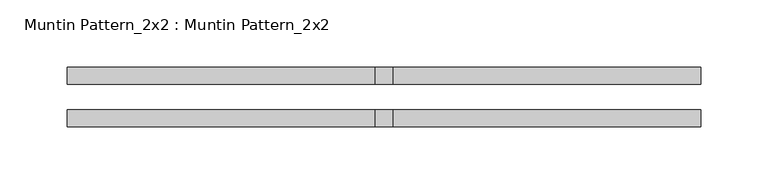
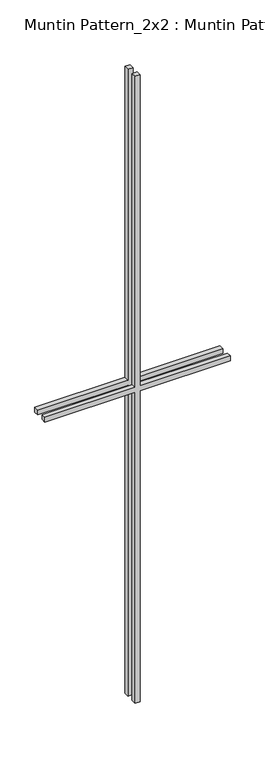
"""IFC4 building model written with IfcOpenShell, lengths in millimetres: proxy geometry, Muntin Pattern_2x2 : Muntin Pattern_2x2."""

from ifc_helpers import new_model, si_unit, frame, origin, place, context, project, spatial, polyline, outline, extrude, source, transform, mapped, element, save


def muntin_pattern_2x2_muntin_pattern_2x2_ef995ed3(model_context):
    return source(origin(), model_context, "Body", "SweptSolid", [
        extrude(outline(polyline([(850.9, -6.35), (850.9, -236.5375), (838.2, -236.5375), (838.2, -6.35), (0.0, -6.35), (0.0, 6.35), (838.2, 6.35), (838.2, 236.5375), (850.9, 236.5375), (850.9, 6.35), (1689.1, 6.35), (1689.1, -6.35), (850.9, -6.35)])), frame((0.0, -22.225, 0.0), z_axis=(0.0, 1.0, 0.0), x_axis=(0.0, 0.0, 1.0)), (0.0, 0.0, 1.0), 12.7),
        extrude(outline(polyline([(850.9, -6.35), (850.9, -236.5375), (838.2, -236.5375), (838.2, -6.35), (0.0, -6.35), (0.0, 6.35), (838.2, 6.35), (838.2, 236.5375), (850.9, 236.5375), (850.9, 6.35), (1689.1, 6.35), (1689.1, -6.35), (850.9, -6.35)])), frame((0.0, 9.525, 0.0), z_axis=(0.0, 1.0, 0.0), x_axis=(0.0, 0.0, 1.0)), (0.0, 0.0, 1.0), 12.7),
    ])


if __name__ == "__main__":
    model = new_model("IFC4")
    model_context = context("Model", 3, world=origin())
    ifc_project = project(units=[si_unit("LENGTHUNIT", "METRE", prefix="MILLI")], contexts=[model_context])
    site = spatial("IfcSite", under=ifc_project)
    building = spatial("IfcBuilding", under=site)
    placement = place(None, origin())
    muntin_pattern_2x2_muntin_pattern_2x2_shape = muntin_pattern_2x2_muntin_pattern_2x2_ef995ed3(model_context)
    element("IfcBuildingElementProxy", 1, Name="Muntin Pattern_2x2 : Muntin Pattern_2x2", ObjectType="Muntin Pattern_2x2 : Muntin Pattern_2x2", at=placement, inside=building, context=model_context, shape_type="MappedRepresentation", body=[
        mapped(muntin_pattern_2x2_muntin_pattern_2x2_shape, transform((0.0, 0.0, 0.0), x_axis=(1.0, 0.0, 0.0), y_axis=(0.0, 1.0, 0.0), z_axis=(0.0, 0.0, 1.0))),
    ])
    save(model, "model.ifc")

# Revit data of these elements
# Type "Muntin Pattern_2x2 : Muntin Pattern_2x2"
#   Width [instance default] = 4' - 0"
#   Thickness = 0' - 0 1/2"
#   Height [instance default] = 4' - 0"
#   Distance = 0' - 0 3/4"
#   Interior Material [instance default] = none
#   Exterior Material [instance default] = none
#   Default Elevation = 0
# Element 1 (IfcBuildingElementProxy, "Muntin Pattern_2x2 : Muntin Pattern_2x2")
#   Width = 1' - 6 5/8"
#   Height = 5' - 6 1/2"
#   Interior Material = Wood - Stained
#   Exterior Material = Clad - White
#   Materials on its faces: "Clad - White", "Wood - Stained"
# Materials
#   "Clad - White": class "Wood", colour RGB 242 242 238, transparency 0, Cost = 0
#   "Wood - Stained": class "Wood", colour RGB 224 178 126, transparency 0, Cost = 0
